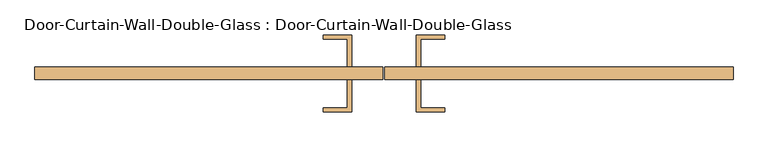
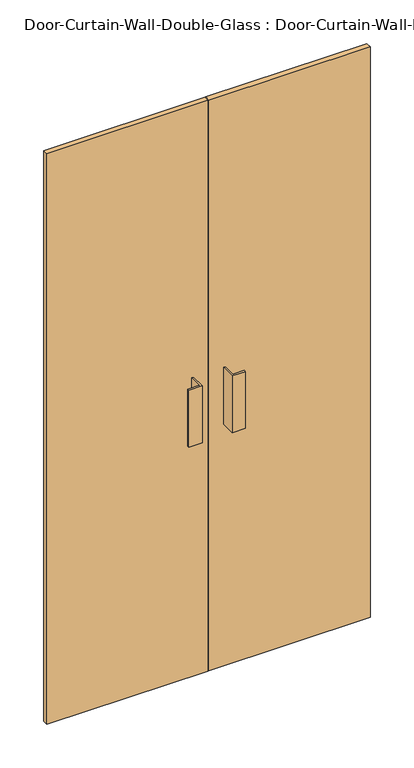
"""IFC4 building model written with IfcOpenShell, lengths in millimetres: door geometry, Door-Curtain-Wall-Double-Glass : Door-Curtain-Wall-Double-Glass."""

from ifc_helpers import new_model, si_unit, frame, origin, origin_with_axes, place, context, project, spatial, polyline, outline, extrude, source, transform, mapped, element, save


def door_curtain_wall_double_glass_door_curtain_wall_double_295e6296(model_context):
    return source(origin(), model_context, "Body", "SweptSolid", [
        extrude(outline(polyline([(546.1, 31.75), (1.5606001, 31.75), (1.5606001, 50.8), (546.1, 50.8), (546.1, 31.75)])), origin_with_axes(), (0.0, 0.0, 1.0), 2038.35),
        extrude(outline(polyline([(-1.6143999, 31.75), (-546.1, 31.75), (-546.1, 50.8), (-1.6143999, 50.8), (-1.6143999, 31.75)])), origin_with_axes(), (0.0, 0.0, 1.0), 2038.35),
        extrude(outline(polyline([(-50.8268999, 101.6), (-50.8268999, 50.8), (-57.1768999, 50.8), (-57.1768999, 95.25), (-95.2768999, 95.25), (-95.2768999, 101.6), (-50.8268999, 101.6)])), frame((0.0, 0.0, 863.6), z_axis=(0.0, 0.0, 1.0), x_axis=(1.0, 0.0, 0.0)), (0.0, 0.0, 1.0), 203.2),
        extrude(outline(polyline([(50.7731001, 101.6), (95.2231001, 101.6), (95.2231001, 95.25), (57.1231001, 95.25), (57.1231001, 50.8), (50.7731001, 50.8), (50.7731001, 101.6)])), frame((0.0, 0.0, 863.6), z_axis=(0.0, 0.0, 1.0), x_axis=(1.0, 0.0, 0.0)), (0.0, 0.0, 1.0), 203.2),
        extrude(outline(polyline([(-50.8268999, -19.05), (-95.2768999, -19.05), (-95.2768999, -12.7), (-57.1768999, -12.7), (-57.1768999, 31.75), (-50.8268999, 31.75), (-50.8268999, -19.05)])), frame((0.0, 0.0, 863.6), z_axis=(0.0, 0.0, 1.0), x_axis=(1.0, 0.0, 0.0)), (0.0, 0.0, 1.0), 203.2),
        extrude(outline(polyline([(50.7731001, -19.05), (50.7731001, 31.75), (57.1231001, 31.75), (57.1231001, -12.7), (95.2231001, -12.7), (95.2231001, -19.05), (50.7731001, -19.05)])), frame((0.0, 0.0, 863.6), z_axis=(0.0, 0.0, 1.0), x_axis=(1.0, 0.0, 0.0)), (0.0, 0.0, 1.0), 203.2),
    ])


if __name__ == "__main__":
    model = new_model("IFC4")
    model_context = context("Model", 3, world=origin())
    ifc_project = project(units=[si_unit("LENGTHUNIT", "METRE", prefix="MILLI")], contexts=[model_context])
    site = spatial("IfcSite", under=ifc_project)
    building = spatial("IfcBuilding", under=site)
    placement = place(None, origin())
    door_curtain_wall_double_glass_door_curtain_wall_double_shape = door_curtain_wall_double_glass_door_curtain_wall_double_295e6296(model_context)
    element("IfcDoor", 1, ObjectType="Door-Curtain-Wall-Double-Glass : Door-Curtain-Wall-Double-Glass", at=placement, inside=building, context=model_context, shape_type="MappedRepresentation", body=[
        mapped(door_curtain_wall_double_glass_door_curtain_wall_double_shape, transform((0.0, 0.0, 0.0), x_axis=(1.0, 0.0, 0.0), y_axis=(0.0, 1.0, 0.0), z_axis=(0.0, 0.0, 1.0))),
    ])
    save(model, "model.ifc")

# Revit data of these elements
# Type "Door-Curtain-Wall-Double-Glass : Door-Curtain-Wall-Double-Glass"
#   Type Mark = "16"
#   Assembly Code = "B2030100"
#   Analytic Construction = "<None>"
#   Width [instance default] = 6' - 0"
#   Thermal Resistance (R) = 10.0000 (h·ft²·°F)/BTU
#   Swing Angle [instance default] = 90.00°
#   Panel Width [instance default] = 3' - 0"
#   Offset = 0' - 2"
#   Heat Transfer Coefficient (U) = 0.1000 BTU/(h·ft²·°F)
#   Define Thermal Properties by = 1
#   Function = 1
#   Door Handle Material = Aluminum
#   Glazing = Glass
#   Visual Light Transmittance = 0
#   Solar Heat Gain Coefficient = 0
#   Construction Type Id = ""
# Element 1 (IfcDoor, "Door-Curtain-Wall-Double-Glass : Door-Curtain-Wall-Double-Glass")
#   Width = 3' - 7"
#   Panel Width = 1' - 9 1/2"
#   Materials on its faces: "Aluminum", "Glass"
# Materials
#   "Aluminum": class "Metal", colour RGB 247 247 247, transparency 0, Description = "Aluminum 6061", Cost = 0
#   "Glass": class "Glass", colour RGB 0 128 192, transparency 0.75, Description = "Soda Lime Glass", Cost = 0
